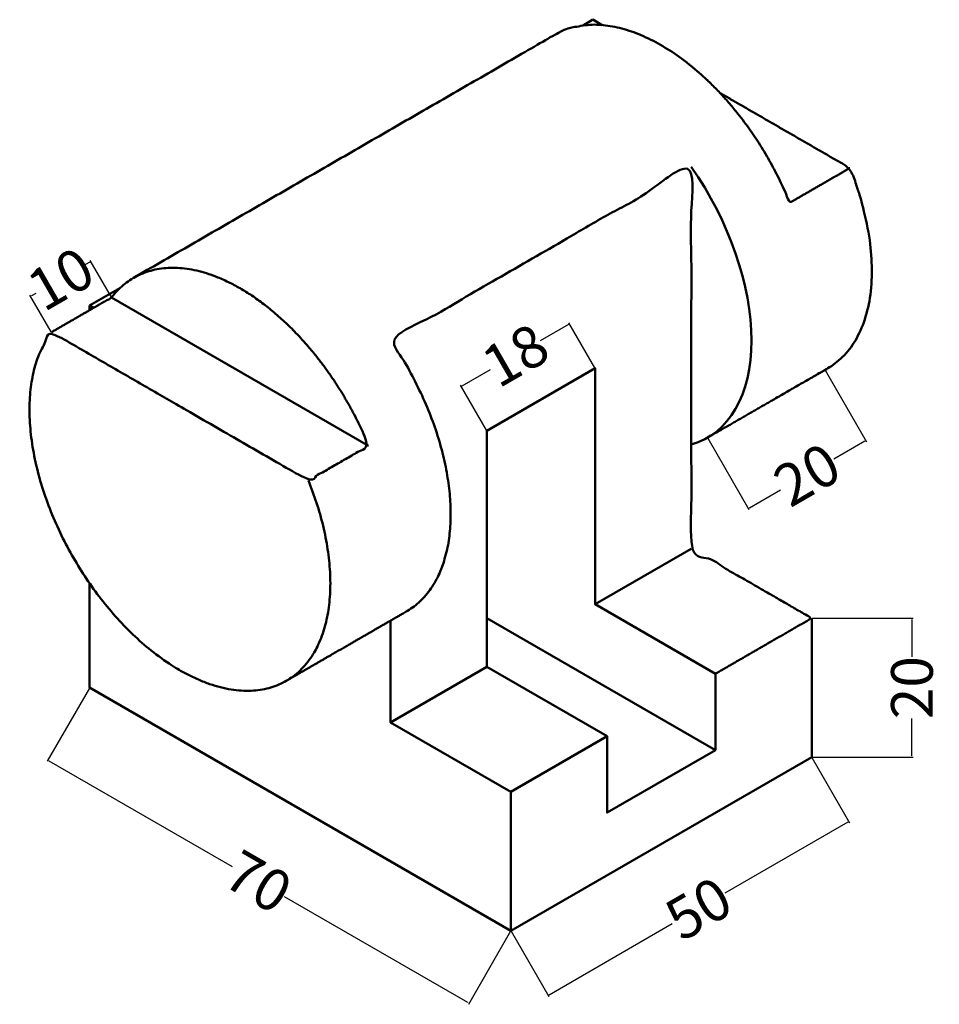
# Model space of a CAD drawing. Units: millimetres. Extents: x -10 to 122, y 17 to 159.
import ezdxf

# ---------------------------------------------------------------- set-up
doc = ezdxf.new("R2010")
doc.units = ezdxf.units.MM
doc.header["$MEASUREMENT"] = 0
doc.layers.add('M-DIMS', color=2, linetype='Continuous', lineweight=25)
doc.layers.add('M-OUTL', color=7, linetype='Continuous', lineweight=50)
doc.styles.get("Standard").update_dxf_attribs({"font": 'arial.ttf'})
doc.dimstyles.get("Standard").update_dxf_attribs({"dimtxt": 6, "dimasz": 0.18, "dimexe": 0.18, "dimexo": 0.0625, "dimgap": 0.09, "dimtad": 0, "dimtoh": 1, "dimdec": 0, "dimzin": 0, "dimdsep": 46, "dimtxsty": 'Standard', "dimcen": 0.09, "dimadec": 0, "dimazin": 0, "dimtfac": 1, "dimtdec": 0, "dimtofl": 0, "dimtmove": 0, "dimatfit": 3, "dimfxl": 1, "dimtolj": 1, "dimtzin": 0, "dimarcsym": 0})

# ---------------------------------------------------------------- blocks, each defined once
blk = doc.blocks.new('*D1')
at = {"layer": 'Defpoints', "color": 0, "transparency": 16777216}
for p in [(68.9, 114.87), (72.58, 108.5), (56.99, 99.5)]:
    blk.add_point(p, dxfattribs=at)
at = {"layer": 'M-DIMS', "color": 0, "lineweight": -2, "transparency": 16777216}
for p, q in [((72.55, 108.55), (68.81, 115.03)), ((68.74, 114.78), (64.67, 112.43)), ((53.47, 105.96), (57.55, 108.31)), ((56.96, 99.55), (53.22, 106.03))]:
    blk.add_line(p, q, dxfattribs=at)
at = {"layer": 'M-DIMS', "color": 0, "transparency": 16777216}
for points in [[(68.73, 114.81), (68.76, 114.75), (68.9, 114.87)], [(53.45, 105.99), (53.48, 105.93), (53.31, 105.87)]]:
    blk.add_solid(points, dxfattribs=at)
at = {"layer": 'M-DIMS', "color": 0, "transparency": 16777216, "insert": (61.11, 110.37), "char_height": 6, "attachment_point": 5, "rotation": 30}
blk.add_mtext('\\A1;18', dxfattribs=at)
blk = doc.blocks.new('*D2')
at = {"layer": 'Defpoints', "color": 0, "transparency": 16777216}
for p in [(-0.01, 123.86), (2.99, 118.68), (-5.67, 113.68)]:
    blk.add_point(p, dxfattribs=at)
at = {"layer": 'M-DIMS', "color": 0, "lineweight": -2, "transparency": 16777216}
for p, q in [((-0.16, 123.77), (-0.79, 123.41)), ((2.96, 118.73), (-0.1, 124.02)), ((-8.51, 118.95), (-7.88, 119.32)), ((-5.7, 113.73), (-8.76, 119.02))]:
    blk.add_line(p, q, dxfattribs=at)
at = {"layer": 'M-DIMS', "color": 0, "transparency": 16777216}
for points in [[(-0.18, 123.8), (-0.15, 123.75), (-0.01, 123.86)], [(-8.52, 118.98), (-8.49, 118.93), (-8.67, 118.86)]]:
    blk.add_solid(points, dxfattribs=at)
at = {"layer": 'M-DIMS', "color": 0, "transparency": 16777216, "insert": (-4.34, 121.36), "char_height": 6, "attachment_point": 5, "rotation": 30}
blk.add_mtext('\\A1;10', dxfattribs=at)
blk = doc.blocks.new('*D3')
at = {"layer": 'Defpoints', "color": 0, "transparency": 16777216}
for p in [(103.76, 72.5), (103.76, 52.5), (118.19, 52.5)]:
    blk.add_point(p, dxfattribs=at)
at = {"layer": 'M-DIMS', "color": 0, "lineweight": -2, "transparency": 16777216}
for p, q in [((103.82, 72.5), (118.37, 72.5)), ((118.19, 72.32), (118.19, 66.93)), ((118.19, 52.68), (118.19, 58.07)), ((103.82, 52.5), (118.37, 52.5))]:
    blk.add_line(p, q, dxfattribs=at)
at = {"layer": 'M-DIMS', "color": 0, "transparency": 16777216}
for points in [[(118.16, 72.32), (118.22, 72.32), (118.19, 72.5)], [(118.16, 52.68), (118.22, 52.68), (118.19, 52.5)]]:
    blk.add_solid(points, dxfattribs=at)
at = {"layer": 'M-DIMS', "color": 0, "transparency": 16777216, "insert": (118.19, 62.5), "char_height": 6, "attachment_point": 5, "rotation": 90}
blk.add_mtext('\\A1;20', dxfattribs=at)
blk = doc.blocks.new('*D4')
at = {"layer": 'Defpoints', "color": 0, "transparency": 16777216}
for p in [(-0.17, 62.5), (60.45, 27.5), (54.43, 17.06)]:
    blk.add_point(p, dxfattribs=at)
at = {"layer": 'M-DIMS', "color": 0, "lineweight": -2, "transparency": 16777216}
for p, q in [((-0.2, 62.44), (-6.28, 51.9)), ((-6.04, 51.97), (20.35, 36.74)), ((54.27, 17.15), (27.89, 32.38)), ((60.42, 27.44), (54.34, 16.9))]:
    blk.add_line(p, q, dxfattribs=at)
at = {"layer": 'M-DIMS', "color": 0, "transparency": 16777216}
for points in [[(-6.02, 52), (-6.05, 51.94), (-6.19, 52.06)], [(54.29, 17.18), (54.26, 17.12), (54.43, 17.06)]]:
    blk.add_solid(points, dxfattribs=at)
at = {"layer": 'M-DIMS', "color": 0, "transparency": 16777216, "insert": (24.12, 34.56), "char_height": 6, "attachment_point": 5, "rotation": 330}
blk.add_mtext('\\A1;70', dxfattribs=at)
blk = doc.blocks.new('*D5')
at = {"layer": 'Defpoints', "color": 0, "transparency": 16777216}
for p in [(103.76, 52.5), (109.12, 43.2), (60.45, 27.5)]:
    blk.add_point(p, dxfattribs=at)
at = {"layer": 'M-DIMS', "color": 0, "lineweight": -2, "transparency": 16777216}
for p, q in [((103.79, 52.44), (109.21, 43.05)), ((108.97, 43.11), (91.26, 32.89)), ((65.98, 18.29), (83.68, 28.52)), ((60.49, 27.44), (65.91, 18.05))]:
    blk.add_line(p, q, dxfattribs=at)
at = {"layer": 'M-DIMS', "color": 0, "transparency": 16777216}
for points in [[(108.95, 43.14), (108.98, 43.09), (109.12, 43.2)], [(65.96, 18.32), (65.99, 18.27), (65.82, 18.2)]]:
    blk.add_solid(points, dxfattribs=at)
at = {"layer": 'M-DIMS', "color": 0, "transparency": 16777216, "insert": (87.47, 30.7), "char_height": 6, "attachment_point": 5, "rotation": 30}
blk.add_mtext('\\A1;50', dxfattribs=at)
blk = doc.blocks.new('*D6')
at = {"layer": 'Defpoints', "color": 0, "transparency": 16777216}
for p in [(105.67, 108.25), (88.75, 98.48), (111.55, 98.06)]:
    blk.add_point(p, dxfattribs=at)
at = {"layer": 'M-DIMS', "color": 0, "lineweight": -2, "transparency": 16777216}
for p, q in [((105.7, 108.19), (111.64, 97.9)), ((88.79, 98.43), (94.73, 88.14)), ((111.4, 97.97), (106.93, 95.39)), ((94.79, 88.38), (99.26, 90.96))]:
    blk.add_line(p, q, dxfattribs=at)
at = {"layer": 'M-DIMS', "color": 0, "transparency": 16777216}
for points in [[(111.38, 98), (111.41, 97.94), (111.55, 98.06)], [(94.78, 88.41), (94.81, 88.36), (94.64, 88.29)]]:
    blk.add_solid(points, dxfattribs=at)
at = {"layer": 'M-DIMS', "color": 0, "transparency": 16777216, "insert": (103.09, 93.18), "char_height": 6, "attachment_point": 5, "rotation": 30}
blk.add_mtext('\\A1;20', dxfattribs=at)

msp = doc.modelspace()

# ---------------------------------------------------------------- linework, layer by layer
at = {"layer": 'M-OUTL'}
for p, q in [((70.85, 157.85), (72.27, 158.68)), ((73.62, 157.9), (72.27, 158.68)), ((-0.17, 117.5), (4.16, 120)), ((39.98, 97.32), (2.99, 118.68)), ((-0.17, 117.5), (-0.17, 116.85)), ((0.39, 117.18), (-0.17, 117.5)), ((89.9, 53.5), (56.99, 72.5))]:
    msp.add_line(p, q, dxfattribs=at)
for points in [[(86.43, 82.5), (72.58, 74.5), (72.58, 108.5), (56.99, 99.5), (56.99, 65.5), (43.13, 57.5), (43.13, 72.14)], [(60.45, 47.5), (60.45, 27.5), (-0.17, 62.5), (-0.17, 77.5)], [(74.31, 55.5), (74.31, 44.5), (89.9, 53.5), (89.9, 64.5), (72.58, 74.5)], [(60.45, 27.5), (103.76, 52.5), (103.76, 72.5)], [(56.99, 65.5), (74.31, 55.5), (60.45, 47.5), (43.13, 57.5)]]:
    msp.add_lwpolyline(points, dxfattribs=at)
msp.add_ellipse((73.44, 125), major_axis=(15.31, -26.52), ratio=0.57735, start_param=6.141288, end_param=7.995879, dxfattribs=at)
for points, weights, knots in [([(109.26, 137.32), (104.93, 134.82), (100.6, 132.32), (95.13, 145.86), (84.68, 153.33), (74.23, 160.81), (66.8, 156.51), (36.48, 139.01), (6.17, 121.51)], [1, 1, 1, 0.899428617285, 1, 0.899428617285, 1, 1, 1], [0, 0, 0, 1, 1, 1.904672, 1.904672, 2.809344, 2.809344, 3.809344, 3.809344, 3.809344]), ([(88.75, 98.48), (93.08, 100.98), (97.41, 103.48), (101.74, 105.98), (106.07, 108.48), (118.11, 115.43), (109.26, 137.32), (99.92, 142.71), (90.59, 148.1)], [1, 1, 1, 1, 1, 0.7862223695, 1, 1, 1], [0, 0, 0, 1, 1, 2, 2, 3.332249, 3.332249, 4.332249, 4.332249, 4.332249]), ([(28.13, 63.48), (32.46, 65.98), (36.79, 68.48), (41.12, 70.98), (45.45, 73.48), (52.44, 77.52), (51.74, 89.3), (51.04, 101.09), (43.13, 112.5), (64.78, 125), (86.43, 137.5), (86.43, 110), (86.43, 82.5), (95.1, 77.5), (103.76, 72.5), (96.83, 68.5), (89.9, 64.5)], [1, 1, 1, 1, 1, 0.909725711784, 1, 0.909725711784, 1, 1, 1, 1, 1, 1, 1, 1, 1], [0, 0, 0, 1, 1, 2, 2, 2.856347, 2.856347, 3.712693, 3.712693, 4.712693, 4.712693, 5.712693, 5.712693, 6.712693, 6.712693, 7.712693, 7.712693, 7.712693]), ([(31.32, 92.32), (40.91, 68.58), (26.87, 62.86), (12.82, 57.15), (-1.22, 79.08), (-15.27, 101.01), (-5.67, 113.68), (12.82, 103), (31.32, 92.32), (35.65, 94.82), (39.98, 97.32), (33.65, 112.97), (21.48, 120), (9.32, 127.02), (2.99, 118.68), (-1.34, 116.18), (-5.67, 113.68)], [1, 0.761039413522, 1, 0.761039413522, 1, 0.761039413522, 1, 1, 1, 1, 1, 0.871779788708, 1, 0.871779788708, 1, 1, 1], [0, 0, 0, 1.411765, 1.411765, 2.82353, 2.82353, 4.235295, 4.235295, 5.235295, 5.235295, 6.235295, 6.235295, 7.25924, 7.25924, 8.283185, 8.283185, 9.283185, 9.283185, 9.283185])]:
    msp.add_rational_spline(points, weights, degree=2, knots=knots, dxfattribs=at)

# ---------------------------------------------------------------- dimensions: what is measured, and where the dimension line sits
at = {"layer": 'M-DIMS'}
for p1, p2, distance, picture, middle in [((-5.67, 113.68), (2.99, 118.68), 5.99, '*D2', (-4.34, 121.36)), ((56.99, 99.5), (72.58, 108.5), 7.36, '*D1', (61.11, 110.37)), ((88.75, 98.48), (105.67, 108.25), -11.76, '*D6', (103.09, 93.18)), ((103.76, 72.5), (103.76, 52.5), 14.44, '*D3', (118.19, 62.5)), ((-0.17, 62.5), (60.45, 27.5), -12.05, '*D4', (24.12, 34.56)), ((60.45, 27.5), (103.76, 52.5), -10.73, '*D5', (87.47, 30.7))]:
    dim = msp.add_aligned_dim(p1=p1, p2=p2, distance=distance, dimstyle='Standard', override={"dimclrd": 0, "dimclre": 0, "dimclrt": 0}, dxfattribs=at)
    dim.commit()
    dim.dimension.update_dxf_attribs({"geometry": picture, "text_midpoint": middle})

doc.saveas('drawing.dxf')
